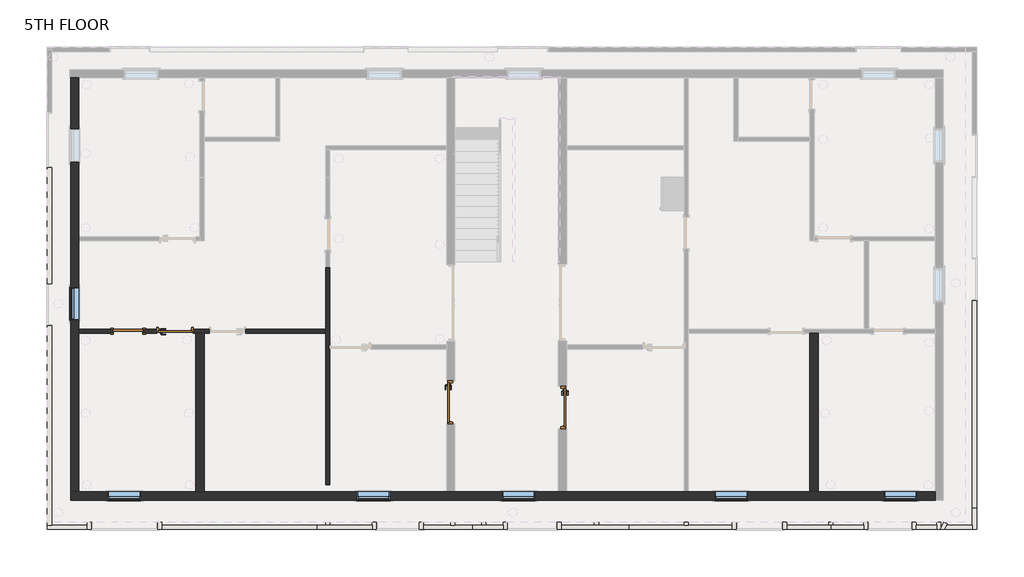
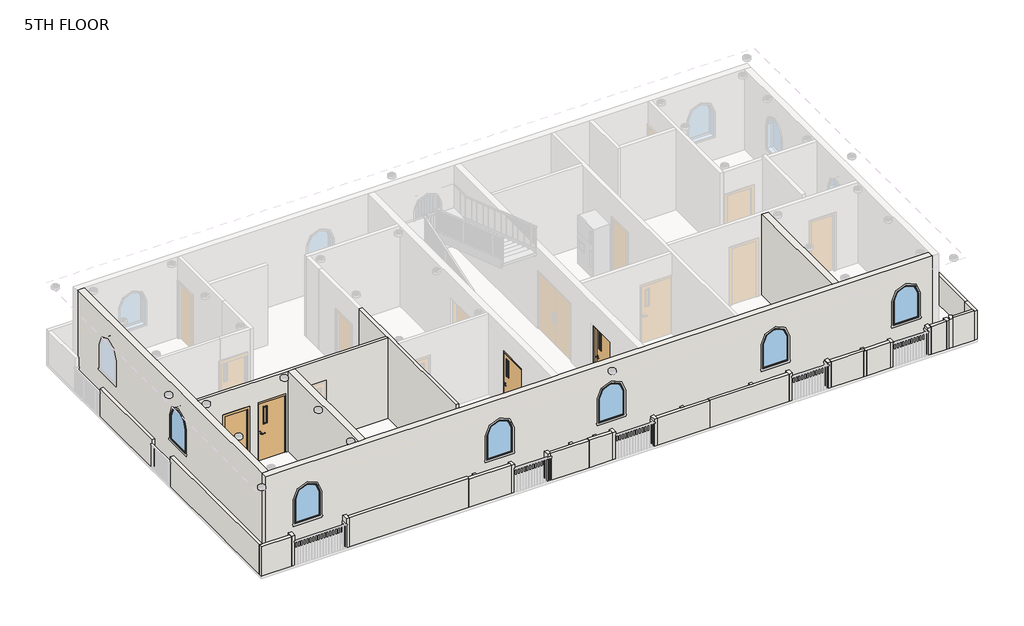
# One storey, part 1 of 7: 39 walls, 6 windows, 4 doors.
# Revit data of these elements (continued)
# Element 4 (IfcDoor, "Single-Flush : 2'8\"x 7'") (continued)
#   Phase Created = New Construction
#   Materials on its faces: "Door - Frame", "Door - Panel"
# Elements 5, 6 (IfcWall, "Generic - 4.5\"")
#   Top Offset = -0' - 6"
#   Base Offset = 0' - 0"
#   wall height = 10' - 0"
#   Phase Created = New Construction
#   Base Constraint = 5TH FLOOR
#   Top Constraint = 6TH FLOOR
#   Materials on its faces: "Default Wall"
# Element 7 (IfcWall, "Generic - 4.5\"")
#   Top Offset = -6' - 10.1834"
#   Base Offset = 0' - 0"
#   wall height = 3' - 7.8166"
#   Phase Created = New Construction
#   Base Constraint = 5TH FLOOR
#   Top Constraint = 6TH FLOOR
#   Materials on its faces: "Default Wall"
# Element 8 (IfcWall, "Generic - 4.5\"")
#   Top Offset = 0' - 0"
#   Base Offset = 0' - 0"
#   Unconnected Height = 3' - 8.64293"
#   wall height = 3' - 8.64293"
#   Phase Created = New Construction
#   Base Constraint = 5TH FLOOR
#   Materials on its faces: "Default Wall"
# Element 9 (IfcWall, "Generic - 4.5\"")
#   Top Offset = -6' - 10.57009"
#   Base Offset = 0' - 0"
#   wall height = 3' - 7.42991"
#   Phase Created = New Construction
#   Base Constraint = 5TH FLOOR
#   Top Constraint = 6TH FLOOR
#   Materials on its faces: "Default Wall"
# Element 10 (IfcWall, "Generic - 4.5\"")
#   Top Offset = -6' - 11.10495"
#   Base Offset = 0' - 0"
#   wall height = 3' - 6.89505"
#   Phase Created = New Construction
#   Base Constraint = 5TH FLOOR
#   Top Constraint = 6TH FLOOR
#   Materials on its faces: "Default Wall"
# Element 11 (IfcWall, "Generic - 4.5\"")
#   Top Offset = -6' - 11.01332"
#   Base Offset = 0' - 0"
#   wall height = 3' - 6.98668"
#   Phase Created = New Construction
#   Base Constraint = 5TH FLOOR
#   Top Constraint = 6TH FLOOR
#   Materials on its faces: "Default Wall"
# Element 12 (IfcWall, "Generic - 4.5\"")
#   Top Offset = -7' - 0.14651"
#   Base Offset = 0' - 0"
#   wall height = 3' - 5.85349"
#   Phase Created = New Construction
#   Base Constraint = 5TH FLOOR
#   Top Constraint = 6TH FLOOR
#   Materials on its faces: "Default Wall"
# Element 13 (IfcWall, "Generic - 4.5\"")
#   Top Offset = -6' - 11.98199"
#   Base Offset = 0' - 0"
#   wall height = 3' - 6.01801"
#   Phase Created = New Construction
#   Base Constraint = 5TH FLOOR
#   Top Constraint = 6TH FLOOR
#   Materials on its faces: "Default Wall"
# Elements 14, 16 (IfcWall, "Generic - 4.5\"")
#   Top Offset = -7' - 2"
#   Base Offset = 0' - 0"
#   wall height = 3' - 4"
#   Phase Created = New Construction
#   Base Constraint = 5TH FLOOR
#   Top Constraint = 6TH FLOOR
#   Materials on its faces: "Default Wall"
# Element 15 (IfcWall, "Generic - 4.5\"")
#   Top Offset = -7' - 1.47546"
#   Base Offset = 0' - 0"
#   wall height = 3' - 4.52454"
#   Phase Created = New Construction
#   Base Constraint = 5TH FLOOR
#   Top Constraint = 6TH FLOOR
#   Materials on its faces: "Default Wall"
# Elements 17, 33, 34 (IfcWall, "Generic - 4.5\"")
#   Top Offset = -7' - 2.10925"
#   Base Offset = 0' - 0"
#   wall height = 3' - 3.89075"
#   Phase Created = New Construction
#   Base Constraint = 5TH FLOOR
#   Top Constraint = 6TH FLOOR
#   Materials on its faces: "Default Wall"
# Elements 18, 19 (IfcWall, "Generic - 4.5\"")
#   Top Offset = -7' - 1.54885"
#   Base Offset = 0' - 0"
#   wall height = 3' - 4.45115"
#   Phase Created = New Construction
#   Base Constraint = 5TH FLOOR
#   Top Constraint = 6TH FLOOR
#   Materials on its faces: "Default Wall"
# Element 20 (IfcWall, "Generic - 4.5\"")
#   Top Offset = -7' - 1.35503"
#   Base Offset = 0' - 0"
#   wall height = 3' - 4.64497"
#   Phase Created = New Construction
#   Base Constraint = 5TH FLOOR
#   Top Constraint = 6TH FLOOR
#   Materials on its faces: "Default Wall"
# Element 21 (IfcWall, "Generic - 4.5\"")
#   Top Offset = -7' - 3.70017"
#   Base Offset = 0' - 0"
#   wall height = 3' - 2.29983"
#   Phase Created = New Construction
#   Base Constraint = 5TH FLOOR
#   Top Constraint = 6TH FLOOR
#   Materials on its faces: "Default Wall"
# Element 22 (IfcWall, "Generic - 4.5\"")
#   Top Offset = -7' - 3.69456"
#   Base Offset = 0' - 0"
#   wall height = 3' - 2.30544"
#   Phase Created = New Construction
#   Base Constraint = 5TH FLOOR
#   Top Constraint = 6TH FLOOR
#   Materials on its faces: "Default Wall"
# Element 23 (IfcWall, "Generic - 4.5\"")
#   Top Offset = -7' - 4.34583"
#   Base Offset = 0' - 0"
#   wall height = 3' - 1.65417"
#   Phase Created = New Construction
#   Base Constraint = 5TH FLOOR
#   Top Constraint = 6TH FLOOR
#   Materials on its faces: "Default Wall"
# Element 24 (IfcWall, "Generic - 4.5\"")
#   Top Offset = -7' - 3.82361"
#   Base Offset = 0' - 0"
#   wall height = 3' - 2.17639"
#   Phase Created = New Construction
#   Base Constraint = 5TH FLOOR
#   Top Constraint = 6TH FLOOR
#   Materials on its faces: "Default Wall"
# Element 25 (IfcWall, "Generic - 4.5\"")
#   Top Offset = -7' - 4.51157"
#   Base Offset = 0' - 0"
#   wall height = 3' - 1.48843"
#   Phase Created = New Construction
#   Base Constraint = 5TH FLOOR
#   Top Constraint = 6TH FLOOR
#   Materials on its faces: "Default Wall"
# Element 26 (IfcWall, "Generic - 4.5\"")
#   Top Offset = -7' - 1.5942"
#   Base Offset = 0' - 0"
#   wall height = 3' - 4.4058"
#   Phase Created = New Construction
#   Base Constraint = 5TH FLOOR
#   Top Constraint = 6TH FLOOR
#   Materials on its faces: "Default Wall"
# Elements 27, 28 (IfcWall, "Generic - 4.5\"")
#   Top Offset = -7' - 0.71294"
#   Base Offset = 0' - 0"
#   wall height = 3' - 5.28706"
#   Phase Created = New Construction
#   Base Constraint = 5TH FLOOR
#   Top Constraint = 6TH FLOOR
#   Materials on its faces: "Default Wall"
# Element 29 (IfcWall, "Generic - 4.5\"")
#   Top Offset = -7' - 0.30229"
#   Base Offset = 0' - 0"
#   wall height = 3' - 5.69771"
#   Phase Created = New Construction
#   Base Constraint = 5TH FLOOR
#   Top Constraint = 6TH FLOOR
#   Materials on its faces: "Default Wall"
# Element 30 (IfcWall, "Generic - 4.5\"")
#   Top Offset = -7' - 1.97028"
#   Base Offset = 0' - 0"
#   wall height = 3' - 4.02972"
#   Phase Created = New Construction
#   Base Constraint = 5TH FLOOR
#   Top Constraint = 6TH FLOOR
#   Materials on its faces: "Default Wall"
# Element 31 (IfcWall, "Generic - 4.5\"")
#   Top Offset = -7' - 1.40393"
#   Base Offset = 0' - 0"
#   wall height = 3' - 4.59607"
#   Phase Created = New Construction
#   Base Constraint = 5TH FLOOR
#   Top Constraint = 6TH FLOOR
#   Materials on its faces: "Default Wall"
# Element 32 (IfcWall, "Generic - 4.5\"")
#   Top Offset = -7' - 1.68978"
#   Base Offset = 0' - 0"
#   wall height = 3' - 4.31022"
#   Phase Created = New Construction
#   Base Constraint = 5TH FLOOR
#   Top Constraint = 6TH FLOOR
#   Materials on its faces: "Default Wall"
# Elements 35, 36 (IfcWall, "Generic - 4.5\"")
#   Top Offset = -6' - 10.38959"
#   Base Offset = 0' - 0"
#   wall height = 3' - 7.61041"
#   Phase Created = New Construction
#   Base Constraint = 5TH FLOOR
#   Top Constraint = 6TH FLOOR
#   Materials on its faces: "Default Wall"
# Element 37 (IfcWall, "Generic - 4.5\"")
#   Top Offset = 0' - 0"
#   Base Offset = 0' - 0"
#   Unconnected Height = 3' - 7.86488"
#   wall height = 3' - 7.86488"
#   Phase Created = New Construction
#   Base Constraint = 5TH FLOOR
#   Materials on its faces: "Default Wall"
# Element 38 (IfcWall, "Generic - 4.5\"")
#   Top Offset = -7' - 0.76215"
#   Base Offset = 0' - 0"
#   wall height = 3' - 5.23785"
#   Phase Created = New Construction
#   Base Constraint = 5TH FLOOR
#   Top Constraint = 6TH FLOOR
#   Materials on its faces: "Default Wall"
# Element 39 (IfcWall, "Generic - 4.5\"")
#   Top Offset = -6' - 11.21767"
#   Base Offset = 0' - 0"
#   wall height = 3' - 6.78233"
#   Phase Created = New Construction
#   Base Constraint = 5TH FLOOR
#   Top Constraint = 6TH FLOOR
#   Materials on its faces: "Default Wall"
# Elements 40, 41, 42, 43 (IfcWall, "Generic - 9\"")
#   Top Offset = -0' - 6"
#   Base Offset = 0' - 0"
#   wall height = 10' - 0"
#   Phase Created = New Construction
#   Base Constraint = 5TH FLOOR
#   Top Constraint = 6TH FLOOR
#   Materials on its faces: "Concrete Masonry Units"
# Element 44 (IfcWindow, "Window-Fixed-Round-Top : 3' x 4'")
#   Mark = "184"
#   Window Inset = 0' - 0"
#   Interior Wall Closure = 0' - 2 1/4"
#   Frame Extension = 0' - 0 1/4"
#   Exterior Wall Closure = 0' - 1 1/4"
#   Interior Trim Visibility = yes
#   Exterior Trim Visibility = yes
#   Phase Created = New Construction
#   Materials on its faces: "Wood - Stained", "Clad - White", "Glass"
# Element 45 (IfcWindow, "Window-Fixed-Round-Top : 3' x 4'")
#   Mark = "185"
#   Window Inset = 0' - 0"
#   Interior Wall Closure = 0' - 2 1/4"
#   Frame Extension = 0' - 0 1/4"
#   Exterior Wall Closure = 0' - 1 1/4"
#   Interior Trim Visibility = yes
#   Exterior Trim Visibility = yes
#   Phase Created = New Construction
#   Materials on its faces: "Wood - Stained", "Clad - White", "Glass"
# Element 46 (IfcWindow, "Window-Fixed-Round-Top : 3' x 4'")
#   Mark = "186"
#   Window Inset = 0' - 0"
#   Interior Wall Closure = 0' - 2 1/4"
#   Frame Extension = 0' - 0 1/4"
#   Exterior Wall Closure = 0' - 1 1/4"
#   Interior Trim Visibility = yes
#   Exterior Trim Visibility = yes
#   Phase Created = New Construction
#   Materials on its faces: "Wood - Stained", "Clad - White", "Glass"
# Element 47 (IfcWindow, "Window-Fixed-Round-Top : 3' x 4'")
#   Mark = "187"
#   Window Inset = 0' - 0"
#   Interior Wall Closure = 0' - 2 1/4"
#   Frame Extension = 0' - 0 1/4"
#   Exterior Wall Closure = 0' - 1 1/4"
#   Interior Trim Visibility = yes
#   Exterior Trim Visibility = yes
#   Phase Created = New Construction
#   Materials on its faces: "Wood - Stained", "Clad - White", "Glass"
# Element 48 (IfcWindow, "Window-Fixed-Round-Top : 3' x 4'")
#   Mark = "188"
#   Window Inset = 0' - 0"
#   Interior Wall Closure = 0' - 2 1/4"
#   Frame Extension = 0' - 0 1/4"
#   Exterior Wall Closure = 0' - 1 1/4"
#   Interior Trim Visibility = yes
#   Exterior Trim Visibility = yes
#   Phase Created = New Construction
#   Materials on its faces: "Wood - Stained", "Clad - White", "Glass"
# Element 49 (IfcWindow, "Window-Fixed-Round-Top : 3' x 4'")
#   Mark = "196"
#   Window Inset = 0' - 0"
#   Interior Wall Closure = 0' - 2 1/4"
#   Frame Extension = 0' - 0 1/4"
#   Exterior Wall Closure = 0' - 1 1/4"
#   Interior Trim Visibility = yes
#   Exterior Trim Visibility = yes
#   Phase Created = New Construction
#   Materials on its faces: "Wood - Stained", "Clad - White", "Glass"
# Materials
#   "Wood - Birch": class "Wood", colour RGB 166 116 52, transparency 0, Cost = 0
#   "Glass": class "Glass", colour RGB 0 128 192, transparency 0.75, Description = "Soda Lime Glass", Cost = 0
#   "Metal - Paint Finish - Grey": class "Paint", colour RGB 104 104 104, transparency 0, Cost = 0
#   "Aluminum": class "Metal", colour RGB 247 247 247, transparency 0, Description = "Aluminum 6061", Cost = 0
#   "Door - Panel": class "Wood", colour RGB 210 159 95, transparency 0, Cost = 0
#   "Door - Frame": colour RGB 118 70 51, transparency 0, Cost = 0
#   "Concrete Masonry Units": class "Masonry", colour RGB 227 227 227, transparency 0, Description = "Concrete masonry units", Cost = 0
#   "Wood - Stained": class "Wood", colour RGB 224 178 126, transparency 0, Cost = 0
#   "Clad - White": class "Wood", colour RGB 242 242 238, transparency 0, Cost = 0
#   "Default Wall": colour RGB 128 128 128, transparency 0, Cost = 0
